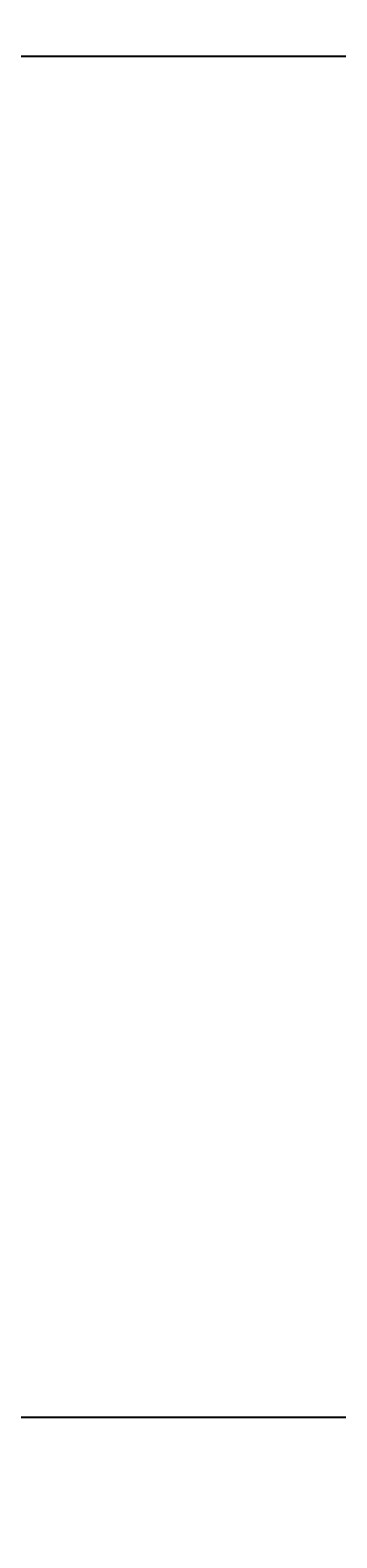
# Model space of a CAD drawing. Units: inches. Extents: x 35362 to 73946, y 43607 to 67532.
# Tile 46 of 134: x 48437 to 48533, y 46091 to 46564. Entities that reach past the tile are written whole.
import ezdxf

# ---------------------------------------------------------------- set-up
doc = ezdxf.new("R2010")
doc.units = ezdxf.units.IN
doc.header["$MEASUREMENT"] = 0
doc.layers.add('A-ANNO-DIMS', color=2, linetype='Continuous', lineweight=18)
doc.styles.get("Standard").update_dxf_attribs({"font": 'arial.ttf'})
doc.dimstyles.get("Standard").update_dxf_attribs({"dimtxt": 0.18, "dimasz": 0.18, "dimexe": 0.18, "dimexo": 0.0625, "dimgap": 0.09, "dimtad": 0, "dimtih": 1, "dimtoh": 1, "dimdec": 4, "dimzin": 0, "dimdsep": 46, "dimtxsty": 'Standard', "dimcen": 0.09, "dimadec": 0, "dimazin": 0, "dimtfac": 1, "dimtdec": 4, "dimtofl": 0, "dimtmove": 0, "dimatfit": 3, "dimfxl": 1, "dimtolj": 1, "dimtzin": 0, "dimarcsym": 0})

# ---------------------------------------------------------------- blocks, each defined once
blk = doc.blocks.new('*D5')
at = {"layer": 'A-ANNO-DIMS', "color": 0, "lineweight": -2, "transparency": 16777216}
for p, q in [((37121.95, 46919.32), (37121.95, 43606.68)), ((69871.5, 45449.83), (69871.5, 43606.68)), ((37122.13, 43606.86), (53496.29, 43606.86)), ((69871.32, 43606.86), (53497.15, 43606.86))]:
    blk.add_line(p, q, dxfattribs=at)
at = {"layer": 'A-ANNO-DIMS', "color": 0, "transparency": 16777216}
for points in [[(37122.13, 43606.89), (37122.13, 43606.83), (37121.95, 43606.86)], [(69871.32, 43606.89), (69871.32, 43606.83), (69871.5, 43606.86)]]:
    blk.add_solid(points, dxfattribs=at)
at = {"layer": 'Defpoints', "color": 0, "transparency": 16777216}
for p in [(37121.95, 46919.38), (69871.5, 45449.89), (69871.5, 43606.86)]:
    blk.add_point(p, dxfattribs=at)
at = {"layer": 'A-ANNO-DIMS', "color": 0, "transparency": 16777216, "insert": (53496.72, 43606.86), "char_height": 0.18, "attachment_point": 5}
blk.add_mtext('\\A1;32750', dxfattribs=at)
blk = doc.blocks.new('*D11')
at = {"layer": 'A-ANNO-DIMS', "color": 0, "lineweight": -2, "transparency": 16777216}
for p, q in [((47978.66, 56028.77), (47978.66, 43606.68)), ((53109.76, 56028.77), (53109.76, 43606.68)), ((47978.84, 43606.86), (50543.87, 43606.86)), ((53109.58, 43606.86), (50544.55, 43606.86))]:
    blk.add_line(p, q, dxfattribs=at)
at = {"layer": 'A-ANNO-DIMS', "color": 0, "transparency": 16777216}
for points in [[(47978.84, 43606.89), (47978.84, 43606.83), (47978.66, 43606.86)], [(53109.58, 43606.89), (53109.58, 43606.83), (53109.76, 43606.86)]]:
    blk.add_solid(points, dxfattribs=at)
at = {"layer": 'Defpoints', "color": 0, "transparency": 16777216}
for p in [(47978.66, 56028.84), (53109.76, 56028.84), (53109.76, 43606.86)]:
    blk.add_point(p, dxfattribs=at)
at = {"layer": 'A-ANNO-DIMS', "color": 0, "transparency": 16777216, "insert": (50544.21, 43606.86), "char_height": 0.18, "attachment_point": 5}
blk.add_mtext('\\A1;5131', dxfattribs=at)
blk = doc.blocks.new('*D13')
at = {"layer": 'A-ANNO-DIMS', "color": 0, "lineweight": -2, "transparency": 16777216}
for p, q in [((48373.49, 51694.02), (48373.49, 43606.68)), ((51029.04, 51694.02), (51029.04, 43606.68)), ((48373.67, 43606.86), (49700.8, 43606.86)), ((51028.86, 43606.86), (49701.73, 43606.86))]:
    blk.add_line(p, q, dxfattribs=at)
at = {"layer": 'A-ANNO-DIMS', "color": 0, "transparency": 16777216}
for points in [[(48373.67, 43606.89), (48373.67, 43606.83), (48373.49, 43606.86)], [(51028.86, 43606.89), (51028.86, 43606.83), (51029.04, 43606.86)]]:
    blk.add_solid(points, dxfattribs=at)
at = {"layer": 'Defpoints', "color": 0, "transparency": 16777216}
for p in [(48373.49, 51694.09), (51029.04, 51694.09), (51029.04, 43606.86)]:
    blk.add_point(p, dxfattribs=at)
at = {"layer": 'A-ANNO-DIMS', "color": 0, "transparency": 16777216, "insert": (49701.27, 43606.86), "char_height": 0.18, "attachment_point": 5}
blk.add_mtext('\\A1;2655.6', dxfattribs=at)
blk = doc.blocks.new('*D67')
at = {"layer": 'A-ANNO-DIMS', "color": 0, "lineweight": -2, "transparency": 16777216}
for p, q in [((56873.54, 53351.53), (35361.77, 53351.53)), ((35361.95, 53351.35), (35361.95, 49400.89)), ((35361.95, 45450.07), (35361.95, 49400.53)), ((53793.58, 45449.89), (35361.77, 45449.89))]:
    blk.add_line(p, q, dxfattribs=at)
at = {"layer": 'A-ANNO-DIMS', "color": 0, "transparency": 16777216}
for points in [[(35361.92, 53351.35), (35361.98, 53351.35), (35361.95, 53351.53)], [(35361.92, 45450.07), (35361.98, 45450.07), (35361.95, 45449.89)]]:
    blk.add_solid(points, dxfattribs=at)
at = {"layer": 'Defpoints', "color": 0, "transparency": 16777216}
for p in [(35361.95, 53351.53), (56873.6, 53351.53), (53793.64, 45449.89)]:
    blk.add_point(p, dxfattribs=at)
at = {"layer": 'A-ANNO-DIMS', "color": 0, "transparency": 16777216, "insert": (35361.95, 49400.71), "char_height": 0.18, "attachment_point": 5}
blk.add_mtext('\\A1;7901.6', dxfattribs=at)
blk = doc.blocks.new('*D76')
at = {"layer": 'A-ANNO-DIMS', "color": 0, "lineweight": -2, "transparency": 16777216}
for p, q in [((54052.84, 46555.29), (35361.77, 46555.29)), ((35361.95, 46555.11), (35361.95, 46342.27)), ((35361.95, 46129.06), (35361.95, 46341.9)), ((53793.58, 46128.88), (35361.77, 46128.88))]:
    blk.add_line(p, q, dxfattribs=at)
at = {"layer": 'A-ANNO-DIMS', "color": 0, "transparency": 16777216}
for points in [[(35361.92, 46555.11), (35361.98, 46555.11), (35361.95, 46555.29)], [(35361.92, 46129.06), (35361.98, 46129.06), (35361.95, 46128.88)]]:
    blk.add_solid(points, dxfattribs=at)
at = {"layer": 'Defpoints', "color": 0, "transparency": 16777216}
for p in [(35361.95, 46555.29), (54052.9, 46555.29), (53793.64, 46128.88)]:
    blk.add_point(p, dxfattribs=at)
at = {"layer": 'A-ANNO-DIMS', "color": 0, "transparency": 16777216, "insert": (35361.95, 46342.09), "char_height": 0.18, "attachment_point": 5}
blk.add_mtext('\\A1;426.4', dxfattribs=at)
blk = doc.blocks.new('*D90')
at = {"layer": 'A-ANNO-DIMS', "color": 0, "lineweight": -2, "transparency": 16777216}
for p, q in [((53707.72, 47291.29), (35361.77, 47291.29)), ((35361.95, 47291.11), (35361.95, 46710.26)), ((35361.95, 46129.06), (35361.95, 46709.9)), ((53793.58, 46128.88), (35361.77, 46128.88))]:
    blk.add_line(p, q, dxfattribs=at)
at = {"layer": 'A-ANNO-DIMS', "color": 0, "transparency": 16777216}
for points in [[(35361.92, 47291.11), (35361.98, 47291.11), (35361.95, 47291.29)], [(35361.92, 46129.06), (35361.98, 46129.06), (35361.95, 46128.88)]]:
    blk.add_solid(points, dxfattribs=at)
at = {"layer": 'Defpoints', "color": 0, "transparency": 16777216}
for p in [(53707.78, 47291.29), (35361.95, 46128.88), (53793.64, 46128.88)]:
    blk.add_point(p, dxfattribs=at)
at = {"layer": 'A-ANNO-DIMS', "color": 0, "transparency": 16777216, "insert": (35361.95, 46710.08), "char_height": 0.18, "attachment_point": 5}
blk.add_mtext('\\A1;1162.4', dxfattribs=at)

msp = doc.modelspace()

# ---------------------------------------------------------------- dimensions: what is measured, and where the dimension line sits
at = {"layer": 'A-ANNO-DIMS'}
for base, p1, p2, override, picture, middle in [((53109.76, 43606.859), (47978.665, 56028.836), (53109.76, 56028.836), {"dimdec": 0, "dimlfac": 1, "dimrnd": 0, "dimzin": 0, "dimdsep": 46, "dimlunit": 2}, '*D11', (50544.212, 43606.859)), ((51029.043, 43606.859), (48373.492, 51694.087), (51029.043, 51694.087), {"dimdec": 1, "dimlfac": 1, "dimrnd": 0, "dimzin": 0, "dimdsep": 46, "dimlunit": 2}, '*D13', (49701.267, 43606.859)), ((69871.496, 43606.859), (37121.949, 46919.381), (69871.496, 45449.894), {"dimdec": 0, "dimlfac": 1, "dimrnd": 0, "dimzin": 0, "dimdsep": 46, "dimlunit": 2}, '*D5', (53496.723, 43606.859))]:
    dim = msp.add_linear_dim(base=base, p1=p1, p2=p2, dimstyle='Standard', override=override, dxfattribs=at)
    dim.commit()
    dim.dimension.update_dxf_attribs({"geometry": picture, "text_midpoint": middle})
for base, p1, p2, picture, middle in [((35361.949, 53351.529), (53793.638, 45449.894), (56873.602, 53351.529), '*D67', (35361.949, 49400.712)), ((35361.949, 46128.878), (53707.781, 47291.285), (53793.638, 46128.878), '*D90', (35361.949, 46710.081)), ((35361.949, 46555.293), (53793.638, 46128.878), (54052.899, 46555.293), '*D76', (35361.949, 46342.086))]:
    dim = msp.add_linear_dim(base=base, p1=p1, p2=p2, angle=90, dimstyle='Standard', override={"dimdec": 1, "dimlfac": 1, "dimrnd": 0, "dimzin": 0, "dimdsep": 46, "dimlunit": 2}, dxfattribs=at)
    dim.commit()
    dim.dimension.update_dxf_attribs({"geometry": picture, "text_midpoint": middle})

doc.saveas('drawing.dxf')
